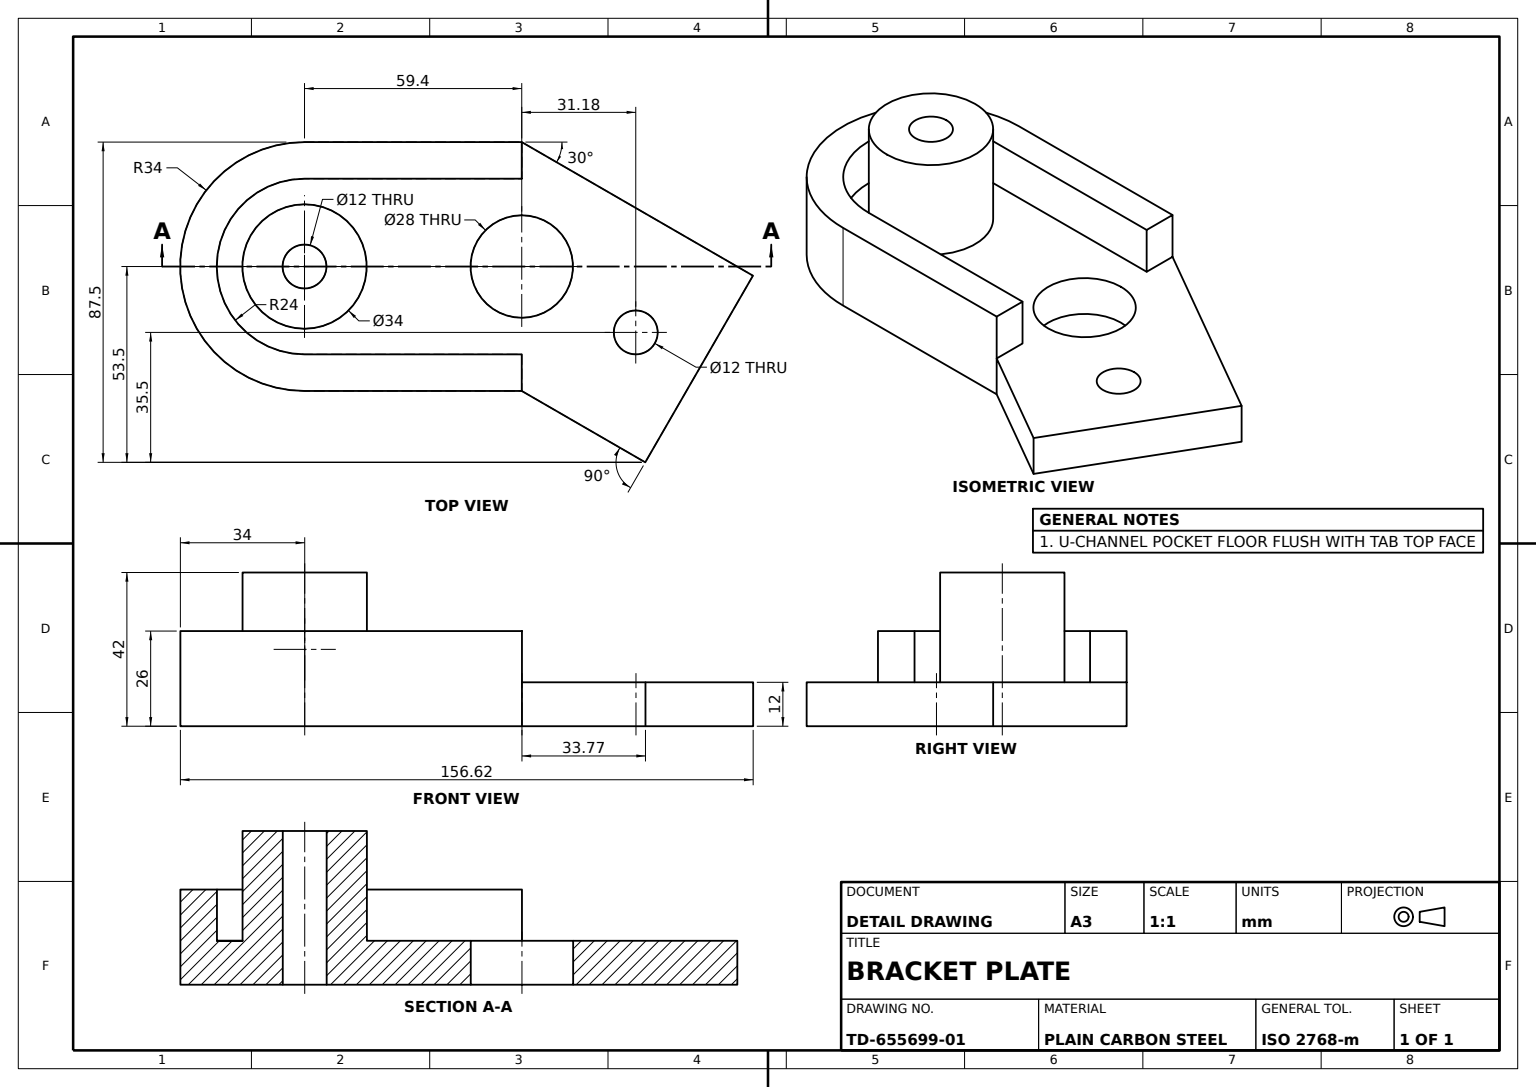
from build123d import *

# Parameters (mm, degrees)
BASE_PLATE_DEPTH          = 26
U_POCKET_14_DEEP_DEPTH    = 14
ANGLED_TAB_30DEG_DEPTH    = 12
BOSS_CIRCLE_SKETCH_R      = 17
BOSS_34_DEPTH             = 30
BOSS_BORE_SKETCH_R        = 6
BOSS_BORE_12_DEPTH        = 141.220821249
TAB_HOLES_SKETCH_R        = 14
TAB_HOLES_SKETCH_R_2      = 6
TAB_HOLES_28_AND_12_DEPTH = 30


with BuildPart() as part:
    # Base Profile Sketch → Base Plate (new body)
    with BuildSketch(Plane(origin=(0, 0, 0), x_dir=(1, 0, 0), z_dir=(0, 1, 0))):
        with BuildLine():
            Line((0, 34), (59.4, 34))
            Line((59.4, 34), (59.4, -34))
            Line((59.4, -34), (0, -34))
            ThreePointArc((0, -34), (-34, 0), (0, 34))
        make_face()
    extrude(amount=BASE_PLATE_DEPTH)

    # Pocket Profile Sketch → U Pocket 14 Deep (cut)
    with BuildSketch(Plane(origin=(0, 26, 0), x_dir=(1, 0, 0), z_dir=(0, 1, 0))):
        with BuildLine():
            Line((0, 24), (59.4, 24))
            Line((59.4, 24), (59.4, -24))
            Line((59.4, -24), (0, -24))
            ThreePointArc((0, -24), (-24, 0), (0, 24))
        make_face()
    extrude(amount=-U_POCKET_14_DEEP_DEPTH, mode=Mode.SUBTRACT)

    # Angled Tab Sketch → Angled Tab 30deg (add)
    with BuildSketch(Plane(origin=(0, 12, 0), x_dir=(1, 0, 0), z_dir=(0, 1, 0))):
        Polygon((59.4, 34), (122.619854476, -2.5), (93.174990748, -53.5), (59.4, -34), align=None)
    extrude(amount=-ANGLED_TAB_30DEG_DEPTH)

    # Boss Circle Sketch → Boss Ø34 (add)
    with BuildSketch(Plane(origin=(0, 12, 0), x_dir=(1, 0, 0), z_dir=(0, 1, 0))):
        with Locations(Location((0, 0, 0), (0, 0, 270))):
            Circle(BOSS_CIRCLE_SKETCH_R)
    extrude(amount=BOSS_34_DEPTH)

    # Boss Bore Sketch → Boss Bore Ø12 (cut, through all)
    with BuildSketch(Plane(origin=(0, 42, 0), x_dir=(1, 0, 0), z_dir=(0, 1, 0))):
        with Locations(Location((0, 0, 0), (0, 0, 270))):
            Circle(BOSS_BORE_SKETCH_R)
    extrude(amount=-BOSS_BORE_12_DEPTH, mode=Mode.SUBTRACT)

    # Tab Holes Sketch → Tab Holes Ø28 and Ø12 (cut)
    with BuildSketch(Plane(origin=(0, 12, 0), x_dir=(1, 0, 0), z_dir=(0, 1, 0))):
        with Locations(Location((59.4, 0, 0), (0, 0, 270))):
            Circle(TAB_HOLES_SKETCH_R)
        with Locations(Location((90.576914536, -18, 0), (0, 0, 270))):
            Circle(TAB_HOLES_SKETCH_R_2)
    extrude(amount=-TAB_HOLES_28_AND_12_DEPTH, mode=Mode.SUBTRACT)


solid = part.part
